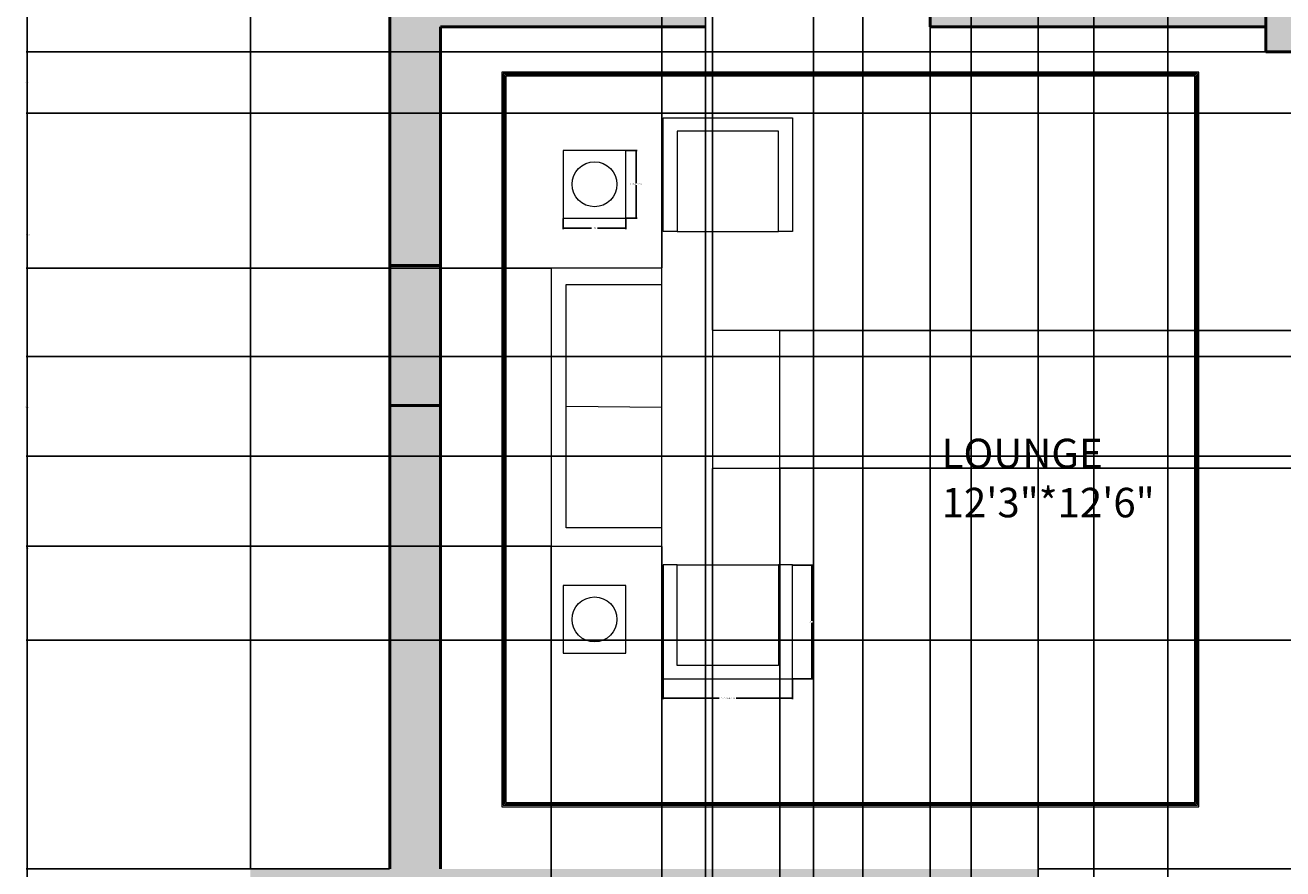
# Model space of a CAD drawing. Units: inches. Extents: x 2494 to 2908, y 1051 to 1885.
# Tile 4 of 7: x 2494 to 2718, y 1457 to 1607. Entities that reach past the tile are written whole.
import ezdxf

# ---------------------------------------------------------------- set-up
doc = ezdxf.new("R2010")
doc.units = ezdxf.units.IN
for name, color, linetype, lineweight in [('A-ANNO-DIMS', 2, 'Continuous', 18), ('A-AREA-IDEN', 130, 'Continuous', 18), ('A-COLS-PATT', 200, 'Continuous', 13), ('A-WALL-PATT', 140, 'Continuous', 13), ('COLUMN', 200, 'Continuous', 50), ('DOOR', 50, 'Continuous', 25), ('FUR', 230, 'Continuous', 18), ('WALL', 140, 'Continuous', 50)]:
    doc.layers.add(name, color=color, linetype=linetype, lineweight=lineweight)
doc.styles.get("Standard").update_dxf_attribs({"font": 'arial.ttf'})
doc.dimstyles.get("Standard").update_dxf_attribs({"dimtxt": 0.18, "dimasz": 0.18, "dimexe": 0.18, "dimexo": 0.0625, "dimgap": 0.09, "dimtad": 0, "dimtih": 1, "dimtoh": 1, "dimdec": 4, "dimzin": 0, "dimdsep": 46, "dimtxsty": 'Standard', "dimcen": 0.09, "dimadec": 0, "dimazin": 0, "dimtfac": 1, "dimtdec": 4, "dimtofl": 0, "dimtmove": 0, "dimatfit": 3, "dimfxl": 1, "dimtolj": 1, "dimtzin": 0, "dimarcsym": 0})

# ---------------------------------------------------------------- blocks, each defined once
blk = doc.blocks.new('*U2')
for p, q in [((0, 0), (0, -6)), ((40, 0), (40, -6))]:
    blk.add_line(p, q)
blk.add_lwpolyline([(0, 0), (0, 40), (1.75, 40), (1.75, 0)], close=True)
blk.add_arc((0, 0), 40, 0, 90)
blk = doc.blocks.new('CHAIR-LOUNGE')
for p, q in [((2.5, 20.27), (0, 20.27)), ((0, 20.27), (0, 0)), ((23.04, 20.27), (20.54, 20.27)), ((23.04, 0), (23.04, 20.27)), ((0, 0), (23.04, 0))]:
    blk.add_line(p, q)
blk.add_lwpolyline([(2.5, 20.27), (20.54, 20.27), (20.54, 2.38), (2.5, 2.38)], close=True)
blk = doc.blocks.new('TABLE-LOUNGE-END')
blk.add_lwpolyline([(11.18, 12.06), (0, 12.06), (0, 0), (11.18, 0)], close=True)
blk.add_circle((5.59, 6.03), 4)
blk = doc.blocks.new('*D18')
at = {"layer": 'A-ANNO-DIMS', "color": 0, "lineweight": -2, "transparency": 16777216}
for p, q in [((2607.9, 1490.44), (2607.9, 1486.87)), ((2630.95, 1490.44), (2630.95, 1486.87)), ((2608.08, 1487.05), (2617.91, 1487.05)), ((2630.77, 1487.05), (2620.94, 1487.05))]:
    blk.add_line(p, q, dxfattribs=at)
at = {"layer": 'A-ANNO-DIMS', "color": 0, "lineweight": 100, "transparency": 16777216}
for points in [[(2608.08, 1487.08), (2608.08, 1487.02), (2607.9, 1487.05)], [(2630.77, 1487.08), (2630.77, 1487.02), (2630.95, 1487.05)]]:
    blk.add_solid(points, dxfattribs=at)
at = {"layer": 'Defpoints', "color": 0, "lineweight": 100, "transparency": 16777216}
for p in [(2607.9, 1490.5), (2630.95, 1490.5), (2630.95, 1487.05)]:
    blk.add_point(p, dxfattribs=at)
at = {"layer": 'A-ANNO-DIMS', "color": 0, "transparency": 16777216, "insert": (2619.43, 1487.05), "char_height": 0.18, "attachment_point": 5}
blk.add_mtext('\\A1;LOUNGE CHAIR 23 TYP.', dxfattribs=at)
blk = doc.blocks.new('*D19')
at = {"layer": 'A-ANNO-DIMS', "color": 0, "lineweight": -2, "transparency": 16777216}
for p, q in [((2631.01, 1510.77), (2634.58, 1510.77)), ((2634.4, 1510.59), (2634.4, 1500.82)), ((2634.4, 1490.68), (2634.4, 1500.46)), ((2631.01, 1490.5), (2634.58, 1490.5))]:
    blk.add_line(p, q, dxfattribs=at)
at = {"layer": 'A-ANNO-DIMS', "color": 0, "lineweight": 100, "transparency": 16777216}
for points in [[(2634.37, 1510.59), (2634.43, 1510.59), (2634.4, 1510.77)], [(2634.37, 1490.68), (2634.43, 1490.68), (2634.4, 1490.5)]]:
    blk.add_solid(points, dxfattribs=at)
at = {"layer": 'Defpoints', "color": 0, "lineweight": 100, "transparency": 16777216}
for p in [(2630.95, 1510.77), (2634.4, 1510.77), (2630.95, 1490.5)]:
    blk.add_point(p, dxfattribs=at)
at = {"layer": 'A-ANNO-DIMS', "color": 0, "transparency": 16777216, "insert": (2634.4, 1500.64), "char_height": 0.18, "attachment_point": 5}
blk.add_mtext('\\A1;20 TYP.', dxfattribs=at)
blk = doc.blocks.new('*D20')
at = {"layer": 'A-ANNO-DIMS', "color": 0, "lineweight": -2, "transparency": 16777216}
for p, q in [((2601.35, 1584.61), (2603.28, 1584.61)), ((2603.1, 1584.43), (2603.1, 1578.76)), ((2603.1, 1572.73), (2603.1, 1578.4)), ((2601.35, 1572.55), (2603.28, 1572.55))]:
    blk.add_line(p, q, dxfattribs=at)
at = {"layer": 'A-ANNO-DIMS', "color": 0, "lineweight": 100, "transparency": 16777216}
for points in [[(2603.07, 1584.43), (2603.13, 1584.43), (2603.1, 1584.61)], [(2603.07, 1572.73), (2603.13, 1572.73), (2603.1, 1572.55)]]:
    blk.add_solid(points, dxfattribs=at)
at = {"layer": 'Defpoints', "color": 0, "lineweight": 100, "transparency": 16777216}
for p in [(2601.29, 1584.61), (2603.1, 1584.61), (2601.29, 1572.55)]:
    blk.add_point(p, dxfattribs=at)
at = {"layer": 'A-ANNO-DIMS', "color": 0, "transparency": 16777216, "insert": (2603.1, 1578.58), "char_height": 0.18, "attachment_point": 5}
blk.add_mtext('\\A1;END TABLE 12 TYP.', dxfattribs=at)
blk = doc.blocks.new('*D21')
at = {"layer": 'A-ANNO-DIMS', "color": 0, "lineweight": -2, "transparency": 16777216}
for p, q in [((2590.11, 1572.49), (2590.11, 1570.56)), ((2590.29, 1570.74), (2595.18, 1570.74)), ((2601.11, 1570.74), (2596.22, 1570.74)), ((2601.29, 1572.49), (2601.29, 1570.56))]:
    blk.add_line(p, q, dxfattribs=at)
at = {"layer": 'A-ANNO-DIMS', "color": 0, "lineweight": 100, "transparency": 16777216}
for points in [[(2590.29, 1570.77), (2590.29, 1570.71), (2590.11, 1570.74)], [(2601.11, 1570.77), (2601.11, 1570.71), (2601.29, 1570.74)]]:
    blk.add_solid(points, dxfattribs=at)
at = {"layer": 'Defpoints', "color": 0, "lineweight": 100, "transparency": 16777216}
for p in [(2590.11, 1572.55), (2601.29, 1572.55), (2601.29, 1570.74)]:
    blk.add_point(p, dxfattribs=at)
at = {"layer": 'A-ANNO-DIMS', "color": 0, "transparency": 16777216, "insert": (2595.7, 1570.74), "char_height": 0.18, "attachment_point": 5}
blk.add_mtext('\\A1;11 TYP.', dxfattribs=at)
blk = doc.blocks.new('*D22')
at = {"layer": 'A-ANNO-DIMS', "color": 0, "lineweight": -2, "transparency": 16777216}
for p, q in [((2534.4, 1456.72), (2534.4, 1885.09)), ((2534.58, 1884.91), (2546.43, 1884.91)), ((2559.07, 1884.91), (2547.22, 1884.91)), ((2559.25, 1845.22), (2559.25, 1885.09))]:
    blk.add_line(p, q, dxfattribs=at)
at = {"layer": 'A-ANNO-DIMS', "color": 0, "lineweight": 100, "transparency": 16777216}
for points in [[(2534.58, 1884.94), (2534.58, 1884.88), (2534.4, 1884.91)], [(2559.07, 1884.94), (2559.07, 1884.88), (2559.25, 1884.91)]]:
    blk.add_solid(points, dxfattribs=at)
at = {"layer": 'Defpoints', "color": 0, "lineweight": 100, "transparency": 16777216}
for p in [(2559.25, 1884.91), (2559.25, 1845.16), (2534.4, 1456.66)]:
    blk.add_point(p, dxfattribs=at)
at = {"layer": 'A-ANNO-DIMS', "color": 0, "transparency": 16777216, "insert": (2546.83, 1884.91), "char_height": 0.18, "attachment_point": 5}
blk.add_mtext('\\A1;24.85', dxfattribs=at)
blk = doc.blocks.new('*D27')
at = {"layer": 'A-ANNO-DIMS', "color": 0, "lineweight": -2, "transparency": 16777216}
for p, q in [((2559.19, 1845.16), (2494.47, 1845.16)), ((2494.65, 1844.98), (2494.65, 1651.09)), ((2494.65, 1456.84), (2494.65, 1650.72)), ((2559.19, 1456.66), (2494.47, 1456.66))]:
    blk.add_line(p, q, dxfattribs=at)
at = {"layer": 'A-ANNO-DIMS', "color": 0, "lineweight": 100, "transparency": 16777216}
for points in [[(2494.62, 1844.98), (2494.68, 1844.98), (2494.65, 1845.16)], [(2494.62, 1456.84), (2494.68, 1456.84), (2494.65, 1456.66)]]:
    blk.add_solid(points, dxfattribs=at)
at = {"layer": 'Defpoints', "color": 0, "lineweight": 100, "transparency": 16777216}
for p in [(2494.65, 1845.16), (2559.25, 1845.16), (2559.25, 1456.66)]:
    blk.add_point(p, dxfattribs=at)
at = {"layer": 'A-ANNO-DIMS', "color": 0, "transparency": 16777216, "insert": (2494.65, 1650.91), "char_height": 0.18, "attachment_point": 5}
blk.add_mtext('\\A1;388.5', dxfattribs=at)
blk = doc.blocks.new('*D28')
at = {"layer": 'A-ANNO-DIMS', "color": 0, "lineweight": -2, "transparency": 16777216}
for p, q in [((2534.34, 1456.66), (2494.47, 1456.66)), ((2494.65, 1456.48), (2494.65, 1397.59)), ((2494.65, 1338.34), (2494.65, 1397.22)), ((2534.34, 1338.16), (2494.47, 1338.16))]:
    blk.add_line(p, q, dxfattribs=at)
at = {"layer": 'A-ANNO-DIMS', "color": 0, "lineweight": 100, "transparency": 16777216}
for points in [[(2494.62, 1456.48), (2494.68, 1456.48), (2494.65, 1456.66)], [(2494.62, 1338.34), (2494.68, 1338.34), (2494.65, 1338.16)]]:
    blk.add_solid(points, dxfattribs=at)
at = {"layer": 'Defpoints', "color": 0, "lineweight": 100, "transparency": 16777216}
for p in [(2494.65, 1456.66), (2534.4, 1456.66), (2534.4, 1338.16)]:
    blk.add_point(p, dxfattribs=at)
at = {"layer": 'A-ANNO-DIMS', "color": 0, "transparency": 16777216, "insert": (2494.65, 1397.41), "char_height": 0.18, "attachment_point": 5}
blk.add_mtext('\\A1;118.5', dxfattribs=at)
blk = doc.blocks.new('*D33')
at = {"layer": 'A-ANNO-DIMS', "color": 0, "lineweight": -2, "transparency": 16777216}
for p, q in [((2697.84, 1155.22), (2697.84, 1885.09)), ((2698.02, 1884.91), (2716.38, 1884.91)), ((2735.54, 1884.91), (2717.17, 1884.91)), ((2735.72, 1155.22), (2735.72, 1885.09))]:
    blk.add_line(p, q, dxfattribs=at)
at = {"layer": 'A-ANNO-DIMS', "color": 0, "lineweight": 100, "transparency": 16777216}
for points in [[(2698.02, 1884.94), (2698.02, 1884.88), (2697.84, 1884.91)], [(2735.54, 1884.94), (2735.54, 1884.88), (2735.72, 1884.91)]]:
    blk.add_solid(points, dxfattribs=at)
at = {"layer": 'Defpoints', "color": 0, "lineweight": 100, "transparency": 16777216}
for p in [(2735.72, 1884.91), (2697.84, 1155.16), (2735.72, 1155.16)]:
    blk.add_point(p, dxfattribs=at)
at = {"layer": 'A-ANNO-DIMS', "color": 0, "transparency": 16777216, "insert": (2716.78, 1884.91), "char_height": 0.18, "attachment_point": 5}
blk.add_mtext('\\A1;37.88', dxfattribs=at)
blk = doc.blocks.new('*D34')
at = {"layer": 'A-ANNO-DIMS', "color": 0, "lineweight": -2, "transparency": 16777216}
for p, q in [((2634.69, 1155.22), (2634.69, 1885.09)), ((2634.87, 1884.91), (2665.87, 1884.91)), ((2697.66, 1884.91), (2666.66, 1884.91)), ((2697.84, 1155.22), (2697.84, 1885.09))]:
    blk.add_line(p, q, dxfattribs=at)
at = {"layer": 'A-ANNO-DIMS', "color": 0, "lineweight": 100, "transparency": 16777216}
for points in [[(2634.87, 1884.94), (2634.87, 1884.88), (2634.69, 1884.91)], [(2697.66, 1884.94), (2697.66, 1884.88), (2697.84, 1884.91)]]:
    blk.add_solid(points, dxfattribs=at)
at = {"layer": 'Defpoints', "color": 0, "lineweight": 100, "transparency": 16777216}
for p in [(2697.84, 1884.91), (2634.69, 1155.16), (2697.84, 1155.16)]:
    blk.add_point(p, dxfattribs=at)
at = {"layer": 'A-ANNO-DIMS', "color": 0, "transparency": 16777216, "insert": (2666.26, 1884.91), "char_height": 0.18, "attachment_point": 5}
blk.add_mtext('\\A1;63.15', dxfattribs=at)
blk = doc.blocks.new('*D40')
at = {"layer": 'A-ANNO-DIMS', "color": 0, "lineweight": -2, "transparency": 16777216}
for p, q in [((2615.49, 1606.59), (2615.49, 1051.41)), ((2655.49, 1606.59), (2655.49, 1051.41)), ((2615.67, 1051.59), (2635.27, 1051.59)), ((2655.31, 1051.59), (2635.71, 1051.59))]:
    blk.add_line(p, q, dxfattribs=at)
at = {"layer": 'A-ANNO-DIMS', "color": 0, "lineweight": 100, "transparency": 16777216}
for points in [[(2615.67, 1051.62), (2615.67, 1051.56), (2615.49, 1051.59)], [(2655.31, 1051.62), (2655.31, 1051.56), (2655.49, 1051.59)]]:
    blk.add_solid(points, dxfattribs=at)
at = {"layer": 'Defpoints', "color": 0, "lineweight": 100, "transparency": 16777216}
for p in [(2615.49, 1606.66), (2655.49, 1606.66), (2655.49, 1051.59)]:
    blk.add_point(p, dxfattribs=at)
at = {"layer": 'A-ANNO-DIMS', "color": 0, "transparency": 16777216, "insert": (2635.49, 1051.59), "char_height": 0.18, "attachment_point": 5}
blk.add_mtext('\\A1;40', dxfattribs=at)
blk = doc.blocks.new('*D41')
at = {"layer": 'A-ANNO-DIMS', "color": 0, "lineweight": -2, "transparency": 16777216}
for p, q in [((2684.64, 1347.22), (2684.64, 1885.09)), ((2684.82, 1884.91), (2704.42, 1884.91)), ((2724.46, 1884.91), (2704.86, 1884.91)), ((2724.64, 1347.22), (2724.64, 1885.09))]:
    blk.add_line(p, q, dxfattribs=at)
at = {"layer": 'A-ANNO-DIMS', "color": 0, "lineweight": 100, "transparency": 16777216}
for points in [[(2684.82, 1884.94), (2684.82, 1884.88), (2684.64, 1884.91)], [(2724.46, 1884.94), (2724.46, 1884.88), (2724.64, 1884.91)]]:
    blk.add_solid(points, dxfattribs=at)
at = {"layer": 'Defpoints', "color": 0, "lineweight": 100, "transparency": 16777216}
for p in [(2724.64, 1884.91), (2684.64, 1347.16), (2724.64, 1347.16)]:
    blk.add_point(p, dxfattribs=at)
at = {"layer": 'A-ANNO-DIMS', "color": 0, "transparency": 16777216, "insert": (2704.64, 1884.91), "char_height": 0.18, "attachment_point": 5}
blk.add_mtext('\\A1;40', dxfattribs=at)
blk = doc.blocks.new('*D42')
at = {"layer": 'A-ANNO-DIMS', "color": 0, "lineweight": -2, "transparency": 16777216}
for p, q in [((2674.75, 1347.22), (2674.75, 1885.09)), ((2674.93, 1884.91), (2679.3, 1884.91)), ((2684.46, 1884.91), (2680.09, 1884.91)), ((2684.64, 1347.22), (2684.64, 1885.09))]:
    blk.add_line(p, q, dxfattribs=at)
at = {"layer": 'A-ANNO-DIMS', "color": 0, "lineweight": 100, "transparency": 16777216}
for points in [[(2674.93, 1884.94), (2674.93, 1884.88), (2674.75, 1884.91)], [(2684.46, 1884.94), (2684.46, 1884.88), (2684.64, 1884.91)]]:
    blk.add_solid(points, dxfattribs=at)
at = {"layer": 'Defpoints', "color": 0, "lineweight": 100, "transparency": 16777216}
for p in [(2684.64, 1884.91), (2674.75, 1347.16), (2684.64, 1347.16)]:
    blk.add_point(p, dxfattribs=at)
at = {"layer": 'A-ANNO-DIMS', "color": 0, "transparency": 16777216, "insert": (2679.7, 1884.91), "char_height": 0.18, "attachment_point": 5}
blk.add_mtext('\\A1;9.889', dxfattribs=at)
blk = doc.blocks.new('*D47')
at = {"layer": 'A-ANNO-DIMS', "color": 0, "lineweight": -2, "transparency": 16777216}
for p, q in [((2674.81, 1456.66), (2908.18, 1456.66)), ((2908, 1456.48), (2908, 1444.53)), ((2908, 1432.23), (2908, 1444.17)), ((2674.81, 1432.05), (2908.18, 1432.05))]:
    blk.add_line(p, q, dxfattribs=at)
at = {"layer": 'A-ANNO-DIMS', "color": 0, "lineweight": 100, "transparency": 16777216}
for points in [[(2907.97, 1456.48), (2908.03, 1456.48), (2908, 1456.66)], [(2907.97, 1432.23), (2908.03, 1432.23), (2908, 1432.05)]]:
    blk.add_solid(points, dxfattribs=at)
at = {"layer": 'Defpoints', "color": 0, "lineweight": 100, "transparency": 16777216}
for p in [(2674.75, 1456.66), (2908, 1456.66), (2674.75, 1432.05)]:
    blk.add_point(p, dxfattribs=at)
at = {"layer": 'A-ANNO-DIMS', "color": 0, "transparency": 16777216, "insert": (2908, 1444.35), "char_height": 0.18, "attachment_point": 5}
blk.add_mtext('\\A1;24.606', dxfattribs=at)
blk = doc.blocks.new('*D48')
at = {"layer": 'A-ANNO-DIMS', "color": 0, "lineweight": -2, "transparency": 16777216}
for p, q in [((2534.4, 1456.72), (2534.4, 1885.09)), ((2534.58, 1884.91), (2604.12, 1884.91)), ((2674.57, 1884.91), (2605.03, 1884.91)), ((2674.75, 1456.72), (2674.75, 1885.09))]:
    blk.add_line(p, q, dxfattribs=at)
at = {"layer": 'A-ANNO-DIMS', "color": 0, "lineweight": 100, "transparency": 16777216}
for points in [[(2534.58, 1884.94), (2534.58, 1884.88), (2534.4, 1884.91)], [(2674.57, 1884.94), (2674.57, 1884.88), (2674.75, 1884.91)]]:
    blk.add_solid(points, dxfattribs=at)
at = {"layer": 'Defpoints', "color": 0, "lineweight": 100, "transparency": 16777216}
for p in [(2674.75, 1884.91), (2534.4, 1456.66), (2674.75, 1456.66)]:
    blk.add_point(p, dxfattribs=at)
at = {"layer": 'A-ANNO-DIMS', "color": 0, "transparency": 16777216, "insert": (2604.58, 1884.91), "char_height": 0.18, "attachment_point": 5}
blk.add_mtext('\\A1;140.35', dxfattribs=at)
blk = doc.blocks.new('*D54')
at = {"layer": 'A-ANNO-DIMS', "color": 0, "lineweight": -2, "transparency": 16777216}
for p, q in [((2739.21, 1530.16), (2494.47, 1530.16)), ((2494.65, 1529.98), (2494.65, 1513.94)), ((2494.65, 1497.54), (2494.65, 1513.57)), ((2739.21, 1497.36), (2494.47, 1497.36))]:
    blk.add_line(p, q, dxfattribs=at)
at = {"layer": 'A-ANNO-DIMS', "color": 0, "lineweight": 100, "transparency": 16777216}
for points in [[(2494.62, 1529.98), (2494.68, 1529.98), (2494.65, 1530.16)], [(2494.62, 1497.54), (2494.68, 1497.54), (2494.65, 1497.36)]]:
    blk.add_solid(points, dxfattribs=at)
at = {"layer": 'Defpoints', "color": 0, "lineweight": 100, "transparency": 16777216}
for p in [(2494.65, 1530.16), (2739.28, 1530.16), (2739.28, 1497.36)]:
    blk.add_point(p, dxfattribs=at)
at = {"layer": 'A-ANNO-DIMS', "color": 0, "transparency": 16777216, "insert": (2494.65, 1513.76), "char_height": 0.18, "attachment_point": 5}
blk.add_mtext('\\A1;32.8', dxfattribs=at)
blk = doc.blocks.new('*D57')
at = {"layer": 'A-ANNO-DIMS', "color": 0, "lineweight": -2, "transparency": 16777216}
for p, q in [((2796.19, 1591.24), (2494.47, 1591.24)), ((2494.65, 1591.06), (2494.65, 1569.76)), ((2494.65, 1548.09), (2494.65, 1569.39)), ((2796.19, 1547.91), (2494.47, 1547.91))]:
    blk.add_line(p, q, dxfattribs=at)
at = {"layer": 'A-ANNO-DIMS', "color": 0, "lineweight": 100, "transparency": 16777216}
for points in [[(2494.62, 1591.06), (2494.68, 1591.06), (2494.65, 1591.24)], [(2494.62, 1548.09), (2494.68, 1548.09), (2494.65, 1547.91)]]:
    blk.add_solid(points, dxfattribs=at)
at = {"layer": 'Defpoints', "color": 0, "lineweight": 100, "transparency": 16777216}
for p in [(2494.65, 1591.24), (2796.25, 1591.24), (2796.25, 1547.91)]:
    blk.add_point(p, dxfattribs=at)
at = {"layer": 'A-ANNO-DIMS', "color": 0, "transparency": 16777216, "insert": (2494.65, 1569.57), "char_height": 0.18, "attachment_point": 5}
blk.add_mtext('\\A1;43.324', dxfattribs=at)
blk = doc.blocks.new('*D58')
at = {"layer": 'A-ANNO-DIMS', "color": 0, "lineweight": -2, "transparency": 16777216}
for p, q in [((2796.19, 1602.16), (2494.47, 1602.16)), ((2494.65, 1601.98), (2494.65, 1596.88)), ((2494.65, 1591.42), (2494.65, 1596.51)), ((2796.19, 1591.24), (2494.47, 1591.24))]:
    blk.add_line(p, q, dxfattribs=at)
at = {"layer": 'A-ANNO-DIMS', "color": 0, "lineweight": 100, "transparency": 16777216}
for points in [[(2494.62, 1601.98), (2494.68, 1601.98), (2494.65, 1602.16)], [(2494.62, 1591.42), (2494.68, 1591.42), (2494.65, 1591.24)]]:
    blk.add_solid(points, dxfattribs=at)
at = {"layer": 'Defpoints', "color": 0, "lineweight": 100, "transparency": 16777216}
for p in [(2494.65, 1602.16), (2796.25, 1602.16), (2796.25, 1591.24)]:
    blk.add_point(p, dxfattribs=at)
at = {"layer": 'A-ANNO-DIMS', "color": 0, "transparency": 16777216, "insert": (2494.65, 1596.7), "char_height": 0.18, "attachment_point": 5}
blk.add_mtext('\\A1;10.92', dxfattribs=at)
blk = doc.blocks.new('*D60')
at = {"layer": 'A-ANNO-DIMS', "color": 0, "lineweight": -2, "transparency": 16777216}
for p, q in [((2587.96, 1514.09), (2587.96, 1051.41)), ((2607.71, 1514.09), (2607.71, 1051.41)), ((2588.14, 1051.59), (2597.45, 1051.59)), ((2607.53, 1051.59), (2598.22, 1051.59))]:
    blk.add_line(p, q, dxfattribs=at)
at = {"layer": 'A-ANNO-DIMS', "color": 0, "lineweight": 100, "transparency": 16777216}
for points in [[(2588.14, 1051.62), (2588.14, 1051.56), (2587.96, 1051.59)], [(2607.53, 1051.62), (2607.53, 1051.56), (2607.71, 1051.59)]]:
    blk.add_solid(points, dxfattribs=at)
at = {"layer": 'Defpoints', "color": 0, "lineweight": 100, "transparency": 16777216}
for p in [(2587.96, 1514.15), (2607.71, 1514.15), (2607.71, 1051.59)]:
    blk.add_point(p, dxfattribs=at)
at = {"layer": 'A-ANNO-DIMS', "color": 0, "transparency": 16777216, "insert": (2597.83, 1051.59), "char_height": 0.18, "attachment_point": 5}
blk.add_mtext('\\A1;19.76', dxfattribs=at)
blk = doc.blocks.new('*D61')
at = {"layer": 'A-ANNO-DIMS', "color": 0, "lineweight": -2, "transparency": 16777216}
for p, q in [((2587.89, 1563.66), (2494.47, 1563.66)), ((2494.65, 1563.48), (2494.65, 1539.09)), ((2494.65, 1514.33), (2494.65, 1538.72)), ((2587.89, 1514.15), (2494.47, 1514.15))]:
    blk.add_line(p, q, dxfattribs=at)
at = {"layer": 'A-ANNO-DIMS', "color": 0, "lineweight": 100, "transparency": 16777216}
for points in [[(2494.62, 1563.48), (2494.68, 1563.48), (2494.65, 1563.66)], [(2494.62, 1514.33), (2494.68, 1514.33), (2494.65, 1514.15)]]:
    blk.add_solid(points, dxfattribs=at)
at = {"layer": 'Defpoints', "color": 0, "lineweight": 100, "transparency": 16777216}
for p in [(2494.65, 1563.66), (2587.96, 1563.66), (2587.96, 1514.15)]:
    blk.add_point(p, dxfattribs=at)
at = {"layer": 'A-ANNO-DIMS', "color": 0, "transparency": 16777216, "insert": (2494.65, 1538.91), "char_height": 0.18, "attachment_point": 5}
blk.add_mtext('\\A1;49.51', dxfattribs=at)
blk = doc.blocks.new('*D62')
at = {"layer": 'A-ANNO-DIMS', "color": 0, "lineweight": -2, "transparency": 16777216}
for p, q in [((2616.72, 1527.95), (2616.72, 1051.41)), ((2628.68, 1527.95), (2628.68, 1051.41)), ((2616.9, 1051.59), (2622.25, 1051.59)), ((2628.5, 1051.59), (2623.16, 1051.59))]:
    blk.add_line(p, q, dxfattribs=at)
at = {"layer": 'A-ANNO-DIMS', "color": 0, "lineweight": 100, "transparency": 16777216}
for points in [[(2616.9, 1051.62), (2616.9, 1051.56), (2616.72, 1051.59)], [(2628.5, 1051.62), (2628.5, 1051.56), (2628.68, 1051.59)]]:
    blk.add_solid(points, dxfattribs=at)
at = {"layer": 'Defpoints', "color": 0, "lineweight": 100, "transparency": 16777216}
for p in [(2616.72, 1528.01), (2628.68, 1528.01), (2628.68, 1051.59)]:
    blk.add_point(p, dxfattribs=at)
at = {"layer": 'A-ANNO-DIMS', "color": 0, "transparency": 16777216, "insert": (2622.7, 1051.59), "char_height": 0.18, "attachment_point": 5}
blk.add_mtext('\\A1;11.963', dxfattribs=at)
blk = doc.blocks.new('*D63')
at = {"layer": 'A-ANNO-DIMS', "color": 0, "lineweight": -2, "transparency": 16777216}
for p, q in [((2628.75, 1552.53), (2908.18, 1552.53)), ((2908, 1552.35), (2908, 1540.45)), ((2908, 1528.19), (2908, 1540.09)), ((2628.75, 1528.01), (2908.18, 1528.01))]:
    blk.add_line(p, q, dxfattribs=at)
at = {"layer": 'A-ANNO-DIMS', "color": 0, "lineweight": 100, "transparency": 16777216}
for points in [[(2907.97, 1552.35), (2908.03, 1552.35), (2908, 1552.53)], [(2907.97, 1528.19), (2908.03, 1528.19), (2908, 1528.01)]]:
    blk.add_solid(points, dxfattribs=at)
at = {"layer": 'Defpoints', "color": 0, "lineweight": 100, "transparency": 16777216}
for p in [(2628.68, 1552.53), (2908, 1552.53), (2628.68, 1528.01)]:
    blk.add_point(p, dxfattribs=at)
at = {"layer": 'A-ANNO-DIMS', "color": 0, "transparency": 16777216, "insert": (2908, 1540.27), "char_height": 0.18, "attachment_point": 5}
blk.add_mtext('\\A1;24.523', dxfattribs=at)
blk = doc.blocks.new('*D64')
at = {"layer": 'A-ANNO-DIMS', "color": 0, "lineweight": -2, "transparency": 16777216}
for p, q in [((2607.71, 1563.72), (2607.71, 1885.09)), ((2607.89, 1884.91), (2611.82, 1884.91)), ((2616.54, 1884.91), (2612.61, 1884.91)), ((2616.72, 1552.6), (2616.72, 1885.09))]:
    blk.add_line(p, q, dxfattribs=at)
at = {"layer": 'A-ANNO-DIMS', "color": 0, "lineweight": 100, "transparency": 16777216}
for points in [[(2607.89, 1884.94), (2607.89, 1884.88), (2607.71, 1884.91)], [(2616.54, 1884.94), (2616.54, 1884.88), (2616.72, 1884.91)]]:
    blk.add_solid(points, dxfattribs=at)
at = {"layer": 'Defpoints', "color": 0, "lineweight": 100, "transparency": 16777216}
for p in [(2616.72, 1884.91), (2607.71, 1563.66), (2616.72, 1552.53)]:
    blk.add_point(p, dxfattribs=at)
at = {"layer": 'A-ANNO-DIMS', "color": 0, "transparency": 16777216, "insert": (2612.22, 1884.91), "char_height": 0.18, "attachment_point": 5}
blk.add_mtext('\\A1;9.008', dxfattribs=at)
blk = doc.blocks.new('*D65')
at = {"layer": 'A-ANNO-DIMS', "color": 0, "lineweight": -2, "transparency": 16777216}
for p, q in [((2662.76, 1694.66), (2662.76, 1051.41)), ((2643.46, 1680.73), (2643.46, 1051.41)), ((2643.64, 1051.59), (2652.66, 1051.59)), ((2662.58, 1051.59), (2653.57, 1051.59))]:
    blk.add_line(p, q, dxfattribs=at)
at = {"layer": 'A-ANNO-DIMS', "color": 0, "lineweight": 100, "transparency": 16777216}
for points in [[(2643.64, 1051.62), (2643.64, 1051.56), (2643.46, 1051.59)], [(2662.58, 1051.62), (2662.58, 1051.56), (2662.76, 1051.59)]]:
    blk.add_solid(points, dxfattribs=at)
at = {"layer": 'Defpoints', "color": 0, "lineweight": 100, "transparency": 16777216}
for p in [(2662.76, 1694.72), (2643.46, 1680.79), (2662.76, 1051.59)]:
    blk.add_point(p, dxfattribs=at)
at = {"layer": 'A-ANNO-DIMS', "color": 0, "transparency": 16777216, "insert": (2653.11, 1051.59), "char_height": 0.18, "attachment_point": 5}
blk.add_mtext('\\A1;19.305', dxfattribs=at)

msp = doc.modelspace()

# ---------------------------------------------------------------- hatches: boundary and pattern name
at = {"layer": 'A-COLS-PATT'}
h = msp.add_hatch(color=256, dxfattribs=at)
h.dxf.hatch_style = 1
h.paths.add_polyline_path([(2584.1612, 1845.1561), (2559.2517, 1845.1561), (2559.2517, 1836.1561), (2584.1612, 1836.1561)])
h.paths.add_polyline_path([(2720.7462, 1845.1561), (2695.8368, 1845.1561), (2695.8368, 1836.1561), (2720.7462, 1836.1561)])
h.paths.add_polyline_path([(2868.2517, 1845.1561), (2843.3423, 1845.1561), (2843.3423, 1836.1561), (2868.2517, 1836.1561)])
h.paths.add_polyline_path([(2568.2517, 1728.1561), (2559.2517, 1728.1561), (2559.2517, 1703.2467), (2568.2517, 1703.2467)])
h.paths.add_polyline_path([(2568.2517, 1564.0885), (2559.2517, 1564.0885), (2559.2517, 1539.1791), (2568.2517, 1539.1791)])
h.paths.add_polyline_path([(2868.2517, 1554.4528), (2859.2517, 1554.4528), (2859.2517, 1529.5434), (2868.2517, 1529.5434)])
h.paths.add_polyline_path([(2806.0841, 1611.1561), (2781.1746, 1611.1561), (2781.1746, 1602.1561), (2806.0841, 1602.1561)])
h.paths.add_polyline_path([(2868.0971, 1611.1561), (2843.1877, 1611.1561), (2843.1877, 1602.1561), (2868.0971, 1602.1561)])
h.paths.add_polyline_path([(2584.1612, 1347.1561), (2559.2517, 1347.1561), (2559.2517, 1338.1561), (2584.1612, 1338.1561)])
h.paths.add_polyline_path([(2868.2517, 1347.1561), (2843.3423, 1347.1561), (2843.3423, 1338.1561), (2868.2517, 1338.1561)])
h.paths.add_polyline_path([(2568.2517, 1180.0656), (2559.2517, 1180.0656), (2559.2517, 1155.1561), (2568.2517, 1155.1561)])
h.paths.add_polyline_path([(2584.1612, 1155.1561), (2559.2517, 1155.1561), (2559.2517, 1146.1561), (2584.1612, 1146.1561)])
h.paths.add_polyline_path([(2868.2517, 1155.1561), (2843.3423, 1155.1561), (2843.3423, 1146.1561), (2868.2517, 1146.1561)])
h.paths.add_polyline_path([(2868.2517, 1180.0656), (2859.2517, 1180.0656), (2859.2517, 1155.1561), (2868.2517, 1155.1561)])
at = {"layer": 'A-WALL-PATT'}
h = msp.add_hatch(color=256, dxfattribs=at)
h.dxf.hatch_style = 1
h.paths.add_polyline_path([(2868.2517, 1836.1561), (2859.2517, 1836.1561), (2859.2517, 1611.1561), (2868.2517, 1611.1561)])
h.paths.add_polyline_path([(2715.2517, 1611.1561), (2655.4916, 1611.1561), (2655.4916, 1606.6561), (2715.2517, 1606.6561)])
h.paths.add_polyline_path([(2781.1746, 1611.1561), (2776.9029, 1611.1561), (2715.2517, 1611.1561), (2715.2517, 1606.6561), (2715.2517, 1602.1561), (2781.1746, 1602.1561)])
h.paths.add_polyline_path([(2868.0971, 1602.1561), (2859.2517, 1602.1561), (2859.2517, 1554.4528), (2868.0971, 1554.4528)])
h.paths.add_polyline_path([(2868.2517, 1529.5434), (2859.2517, 1529.5434), (2859.2517, 1347.1561), (2868.2517, 1347.1561)])
h.paths.add_polyline_path([(2868.2517, 1338.1561), (2859.2517, 1338.1561), (2859.2517, 1243.6561), (2868.2517, 1243.6561)])
h.paths.add_polyline_path([(2568.2517, 1338.1561), (2559.2517, 1338.1561), (2559.2517, 1180.0656), (2568.2517, 1180.0656)])
h.paths.add_polyline_path([(2735.7191, 1155.1561), (2697.838, 1155.1561), (2697.838, 1146.1561), (2735.7191, 1146.1561), (2735.7191, 1151.0155)])
h = msp.add_hatch(color=256, dxfattribs=at)
h.dxf.hatch_style = 1
h.paths.add_polyline_path([(2805.2517, 1547.9123), (2796.2517, 1547.9123), (2796.2517, 1530.1561), (2859.2517, 1530.1561), (2859.2517, 1539.1561), (2805.2517, 1539.1561)])
h.paths.add_polyline_path([(2568.2517, 1606.6561), (2615.4916, 1606.6561), (2615.4916, 1611.1561), (2559.2517, 1611.1561), (2559.2517, 1564.0885), (2568.2517, 1564.0885)])
h.paths.add_polyline_path([(2568.2517, 1539.1791), (2559.2517, 1539.1791), (2559.2517, 1456.6561), (2534.4016, 1456.6561), (2534.4016, 1338.1561), (2559.2517, 1338.1561), (2559.2517, 1342.6561), (2543.4016, 1342.6561), (2543.4016, 1452.1561), (2559.2517, 1452.1561), (2568.2517, 1452.1561), (2674.7517, 1452.1561), (2674.7517, 1456.6561), (2568.2517, 1456.6561)])
h.paths.add_polyline_path([(2684.6403, 1347.1561), (2674.7517, 1347.1561), (2584.1612, 1347.1561), (2584.1612, 1338.1561), (2684.6403, 1338.1561), (2684.6403, 1341.1561)])
h.paths.add_polyline_path([(2843.3423, 1347.1561), (2832.3482, 1347.1561), (2832.3482, 1338.1485), (2843.3423, 1338.1485)])
h.paths.add_polyline_path([(2634.6908, 1155.1561), (2584.1612, 1155.1561), (2584.1612, 1146.1561), (2634.6908, 1146.1561)])
h.paths.add_polyline_path([(2783.7833, 1155.1561), (2772.2517, 1155.1561), (2772.2517, 1146.1561), (2783.7833, 1146.1561)])
h.paths.add_polyline_path([(2843.3423, 1155.1561), (2819.0012, 1155.1561), (2811.9091, 1155.1561), (2811.9091, 1146.1561), (2843.3423, 1146.1561)])
h.paths.add_polyline_path([(2868.2517, 1243.6561), (2859.2517, 1243.6561), (2859.2517, 1239.1561), (2859.2517, 1180.0656), (2868.2517, 1180.0656)])

# ---------------------------------------------------------------- linework, layer by layer
at = {"layer": 'COLUMN'}
msp.add_lwpolyline([(2568.2517, 1564.0885), (2568.2517, 1539.1791), (2559.2517, 1539.1791), (2559.2517, 1564.0885)], close=True, dxfattribs=at)
at = {"layer": 'FUR'}
for p, q in [((2590.6216, 1517.4202), (2590.6216, 1560.7128)), ((2590.6216, 1560.7128), (2607.7136, 1560.7128)), ((2590.6216, 1539.0665), (2607.7136, 1538.9052)), ((2607.7136, 1517.4202), (2590.6216, 1517.4202))]:
    msp.add_line(p, q, dxfattribs=at)
for points in [[(2579.1665, 1467.726), (2703.3514, 1467.726), (2703.3514, 1598.5808), (2579.1665, 1598.5808)], [(2579.4165, 1467.976), (2703.1014, 1467.976), (2703.1014, 1598.3308), (2579.4165, 1598.3308)], [(2579.6665, 1468.226), (2702.8514, 1468.226), (2702.8514, 1598.0808), (2579.6665, 1598.0808)], [(2579.9165, 1468.476), (2702.6014, 1468.476), (2702.6014, 1597.8308), (2579.9165, 1597.8308)], [(2587.9553, 1514.1514), (2607.7136, 1514.1514), (2607.7136, 1563.6591), (2587.9553, 1563.6591)], [(2616.7213, 1528.0102), (2628.6843, 1528.0102), (2628.6843, 1552.5335), (2616.7213, 1552.5335)]]:
    msp.add_lwpolyline(points, close=True, dxfattribs=at)
at = {"layer": 'WALL'}
for p, q in [((2559.2517, 1456.6561), (2559.2517, 1611.1561)), ((2568.2517, 1456.6561), (2568.2517, 1606.6561)), ((2568.2517, 1606.6561), (2615.4916, 1606.6561)), ((2655.4916, 1606.6561), (2715.2517, 1606.6561)), ((2715.2517, 1606.6561), (2715.2517, 1602.1561)), ((2719.7517, 1602.1561), (2715.2517, 1602.1561))]:
    msp.add_line(p, q, dxfattribs=at)
for points in [[(2655.4916, 1606.6561), (2715.2517, 1606.6561), (2715.2517, 1611.1561), (2655.4916, 1611.1561)], [(2715.2517, 1602.1561), (2781.1746, 1602.1561), (2781.1746, 1611.1561), (2715.2517, 1611.1561)]]:
    msp.add_lwpolyline(points, close=True, dxfattribs=at)

# ---------------------------------------------------------------- block references
at = {"layer": 'DOOR'}
msp.add_blockref('*U2', (2615.4916, 1612.6561), dxfattribs=at)
at = {"layer": 'FUR', "extrusion": (0, 0, -1), "zscale": -1, "rotation": 180}
msp.add_blockref('CHAIR-LOUNGE', (-2607.905, 1590.4369), dxfattribs=at)
at = {"layer": 'FUR'}
for name, p in [('TABLE-LOUNGE-END', (2590.109, 1572.5478)), ('CHAIR-LOUNGE', (2607.905, 1490.505)), ('TABLE-LOUNGE-END', (2590.109, 1495.058))]:
    msp.add_blockref(name, p, dxfattribs=at)

# ---------------------------------------------------------------- texts
at = {"layer": 'A-AREA-IDEN', "insert": (2657.5291, 1533.2641), "char_height": 5.248177, "attachment_point": 1}
msp.add_mtext_dynamic_manual_height_columns('LOUNGE\\P12\'3"*12\'6"', width=250.978097, gutter_width=26.2409, heights=[0], dxfattribs=at)

# ---------------------------------------------------------------- dimensions: what is measured, and where the dimension line sits
at = {"layer": 'A-ANNO-DIMS'}
for base, p1, p2, override, picture, middle in [((2559.2517, 1884.9061), (2534.4016, 1456.6561), (2559.2517, 1845.1561), {"dimdec": 2, "dimlfac": 1, "dimrnd": 0, "dimzin": 0, "dimdsep": 46, "dimlunit": 2}, '*D22', (2546.8267, 1884.9061)), ((2674.7517, 1884.9061), (2534.4016, 1456.6561), (2674.7517, 1456.6561), {"dimdec": 2, "dimlfac": 1, "dimrnd": 0, "dimzin": 0, "dimdsep": 46, "dimlunit": 2}, '*D48', (2604.5767, 1884.9061)), ((2616.7213, 1884.9061), (2607.7136, 1563.6591), (2616.7213, 1552.5335), {"dimdec": 3, "dimlfac": 1, "dimrnd": 0, "dimzin": 0, "dimdsep": 46, "dimlunit": 2}, '*D64', (2612.2175, 1884.9061)), ((2697.838, 1884.9061), (2634.6908, 1155.1561), (2697.838, 1155.1561), {"dimdec": 2, "dimlfac": 1, "dimrnd": 0, "dimzin": 0, "dimdsep": 46, "dimlunit": 2}, '*D34', (2666.2644, 1884.9061)), ((2684.6403, 1884.9061), (2674.7517, 1347.1561), (2684.6403, 1347.1561), {"dimdec": 3, "dimlfac": 1, "dimrnd": 0, "dimzin": 0, "dimdsep": 46, "dimlunit": 2}, '*D42', (2679.696, 1884.9061)), ((2724.6403, 1884.9061), (2684.6403, 1347.1561), (2724.6403, 1347.1561), {"dimdec": 0, "dimlfac": 1, "dimrnd": 0, "dimzin": 0, "dimdsep": 46, "dimlunit": 2}, '*D41', (2704.6403, 1884.9061)), ((2735.7191, 1884.9061), (2697.838, 1155.1561), (2735.7191, 1155.1561), {"dimdec": 2, "dimlfac": 1, "dimrnd": 0, "dimzin": 0, "dimdsep": 46, "dimlunit": 2}, '*D33', (2716.7785, 1884.9061)), ((2662.7647, 1051.5937), (2643.4597, 1680.7919), (2662.7647, 1694.719), {"dimdec": 3, "dimlfac": 1, "dimrnd": 0, "dimzin": 0, "dimdsep": 46, "dimlunit": 2}, '*D65', (2653.1122, 1051.5937)), ((2655.4916, 1051.5937), (2615.4916, 1606.6561), (2655.4916, 1606.6561), {"dimdec": 0, "dimlfac": 1, "dimrnd": 0, "dimzin": 0, "dimdsep": 46, "dimlunit": 2}, '*D40', (2635.4916, 1051.5937)), ((2628.6843, 1051.5937), (2616.7213, 1528.0102), (2628.6843, 1528.0102), {"dimdec": 3, "dimlfac": 1, "dimrnd": 0, "dimzin": 0, "dimdsep": 46, "dimlunit": 2}, '*D62', (2622.7028, 1051.5937)), ((2607.7136, 1051.5937), (2587.9553, 1514.1514), (2607.7136, 1514.1514), {"dimdec": 2, "dimlfac": 1, "dimrnd": 0, "dimzin": 0, "dimdsep": 46, "dimlunit": 2}, '*D60', (2597.8345, 1051.5937))]:
    dim = msp.add_linear_dim(base=base, p1=p1, p2=p2, dimstyle='Standard', override=override, dxfattribs=at)
    dim.commit()
    dim.dimension.update_dxf_attribs({"geometry": picture, "text_midpoint": middle})
for base, p1, p2, override, picture, middle in [((2494.6516, 1845.1561), (2559.2517, 1456.6561), (2559.2517, 1845.1561), {"dimdec": 1, "dimlfac": 1, "dimrnd": 0, "dimzin": 0, "dimdsep": 46, "dimlunit": 2}, '*D27', (2494.6516, 1650.9061)), ((2494.6516, 1602.1561), (2796.2517, 1591.2367), (2796.2517, 1602.1561), {"dimdec": 2, "dimlfac": 1, "dimrnd": 0, "dimzin": 0, "dimdsep": 46, "dimlunit": 2}, '*D58', (2494.6516, 1596.6964)), ((2494.6516, 1591.2367), (2796.2517, 1547.9123), (2796.2517, 1591.2367), {"dimdec": 3, "dimlfac": 1, "dimrnd": 0, "dimzin": 0, "dimdsep": 46, "dimlunit": 2}, '*D57', (2494.6516, 1569.5745)), ((2494.6516, 1563.6591), (2587.9553, 1514.1514), (2587.9553, 1563.6591), {"dimdec": 2, "dimlfac": 1, "dimrnd": 0, "dimzin": 0, "dimdsep": 46, "dimlunit": 2}, '*D61', (2494.6516, 1538.9052)), ((2908.0017, 1552.5335), (2628.6843, 1528.0102), (2628.6843, 1552.5335), {"dimdec": 3, "dimlfac": 1, "dimrnd": 0, "dimzin": 0, "dimdsep": 46, "dimlunit": 2}, '*D63', (2908.0017, 1540.2719)), ((2494.6516, 1530.1561), (2739.2763, 1497.3573), (2739.2763, 1530.1561), {"dimdec": 1, "dimlfac": 1, "dimrnd": 0, "dimzin": 0, "dimdsep": 46, "dimlunit": 2}, '*D54', (2494.6516, 1513.7567)), ((2494.6516, 1456.6561), (2534.4016, 1338.1561), (2534.4016, 1456.6561), {"dimdec": 1, "dimlfac": 1, "dimrnd": 0, "dimzin": 0, "dimdsep": 46, "dimlunit": 2}, '*D28', (2494.6516, 1397.4061)), ((2908.0017, 1456.6561), (2674.7517, 1432.0498), (2674.7517, 1456.6561), {"dimdec": 3, "dimlfac": 1, "dimrnd": 0, "dimzin": 0, "dimdsep": 46, "dimlunit": 2}, '*D47', (2908.0017, 1444.353))]:
    dim = msp.add_linear_dim(base=base, p1=p1, p2=p2, angle=90, dimstyle='Standard', override=override, dxfattribs=at)
    dim.commit()
    dim.dimension.update_dxf_attribs({"geometry": picture, "text_midpoint": middle})
for base, p1, p2, text, picture, middle in [((2603.1008, 1584.6092), (2601.2916, 1572.5475), (2601.2916, 1584.6092), 'END TABLE <> TYP.', '*D20', (2603.1008, 1578.5783)), ((2634.4041, 1510.7746), (2630.9477, 1490.5047), (2630.9477, 1510.7746), '<> TYP.', '*D19', (2634.4041, 1500.6397))]:
    dim = msp.add_linear_dim(base=base, p1=p1, p2=p2, angle=90, text=text, dimstyle='Standard', override={"dimdec": 0, "dimlfac": 1, "dimrnd": 0, "dimzin": 0, "dimdsep": 46, "dimlunit": 2}, dxfattribs=at)
    dim.commit()
    dim.dimension.update_dxf_attribs({"geometry": picture, "text_midpoint": middle})
for base, p1, p2, text, picture, middle in [((2601.2916, 1570.7383), (2590.1089, 1572.5475), (2601.2916, 1572.5475), '<> TYP.', '*D21', (2595.7003, 1570.7383)), ((2630.9477, 1487.0483), (2607.9049, 1490.5047), (2630.9477, 1490.5047), 'LOUNGE CHAIR <> TYP.', '*D18', (2619.4263, 1487.0483))]:
    dim = msp.add_linear_dim(base=base, p1=p1, p2=p2, text=text, dimstyle='Standard', override={"dimdec": 0, "dimlfac": 1, "dimrnd": 0, "dimzin": 0, "dimdsep": 46, "dimlunit": 2}, dxfattribs=at)
    dim.commit()
    dim.dimension.update_dxf_attribs({"geometry": picture, "text_midpoint": middle})

doc.saveas('drawing.dxf')
